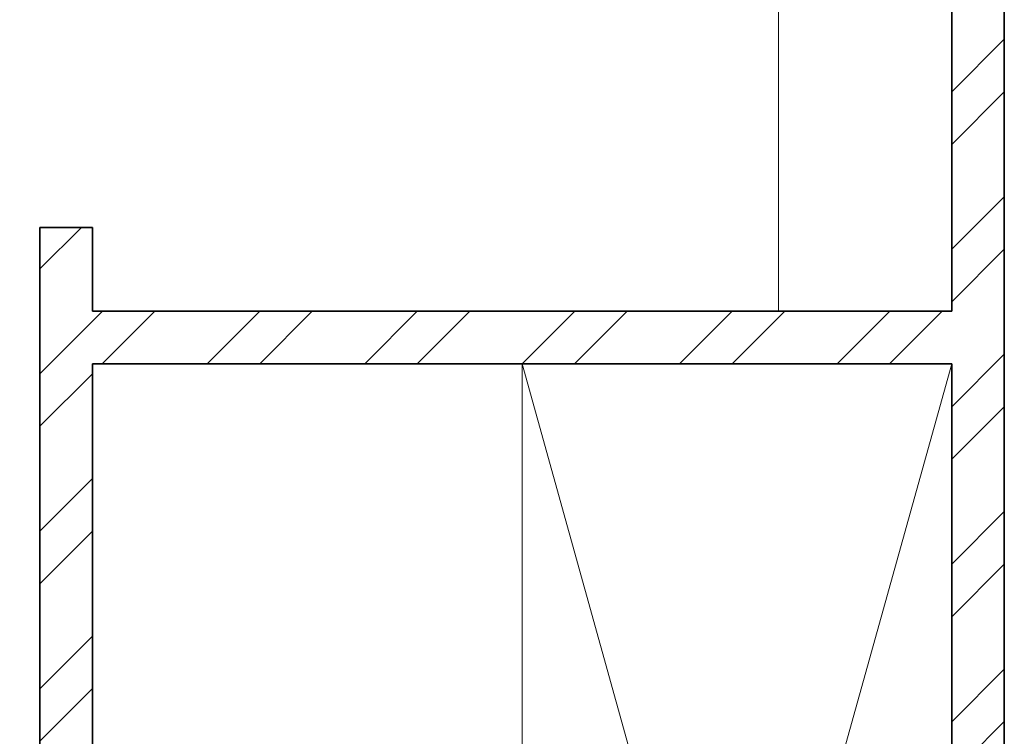
# Model space of a CAD drawing. Units: inches. Extents: x 2168 to 3056, y 1130 to 2629.
# Tile 16 of 42: x 2780 to 2864, y 1956 to 2017. Entities that reach past the tile are written whole.
import ezdxf

# ---------------------------------------------------------------- set-up
doc = ezdxf.new("R2010")
doc.units = ezdxf.units.IN
for name, color, linetype, lineweight in [('A-FLOR-CASE', 71, 'Continuous', 18), ('A-FLOR-OTLN', 7, 'Continuous', 18), ('A-WALL', 7, 'Continuous', 35)]:
    doc.layers.add(name, color=color, linetype=linetype, lineweight=lineweight)
doc.layers.add('A-WALL-PATT', color=143, linetype='Continuous', lineweight=13, true_color=0x7aafdf)

msp = doc.modelspace()

# ---------------------------------------------------------------- hatches: boundary and pattern name
at = {"layer": 'A-WALL-PATT'}
h = msp.add_hatch(dxfattribs=at)
h.set_pattern_fill('ANSI32', color=256)
h.paths.add_polyline_path([(2463.796, 2409.389), (2467.387, 2409.389), (2467.387, 2413.889), (2454.768, 2413.889), (2454.768, 2411.639), (2454.768, 2409.389), (2459.296, 2409.389), (2459.296, 2265.389), (2455.644, 2265.389), (2455.644, 2260.889), (2467.349, 2260.889), (2467.349, 2263.139), (2467.349, 2265.389), (2463.796, 2265.389)])
h.paths.add_polyline_path([(2431.596, 2413.889), (2409.647, 2413.889), (2409.647, 2409.389), (2431.596, 2409.389), (2431.596, 2411.639)])
h.paths.add_polyline_path([(2349.647, 2413.889), (2331.796, 2413.889), (2331.796, 2362.671), (2336.296, 2362.671), (2336.296, 2409.389), (2349.647, 2409.389), (2349.647, 2411.639)])
h.paths.add_polyline_path([(2634.149, 2411.639), (2634.149, 2413.889), (2562.293, 2413.889), (2562.293, 2409.389), (2595.796, 2409.389), (2595.796, 2280.309), (2595.826, 2280.309), (2595.826, 2265.389), (2499.91, 2265.389), (2499.91, 2260.889), (2550.796, 2260.889), (2550.796, 2117.308), (2555.296, 2117.308), (2555.296, 2168.08), (2571.93, 2168.08), (2571.93, 2176.889), (2559.796, 2176.889), (2559.796, 2256.389), (2640.796, 2256.389), (2640.796, 2176.889), (2626.428, 2176.889), (2626.428, 2168.08), (2645.296, 2168.08), (2645.296, 2116.637), (2649.796, 2116.637), (2649.796, 2260.889), (2691.251, 2260.889), (2691.251, 2263.139), (2691.251, 2265.389), (2670.655, 2265.389), (2670.655, 2265.365), (2600.296, 2265.365), (2600.296, 2280.258), (2600.296, 2409.389), (2634.149, 2409.389)])
h.paths.add_polyline_path([(2600.296, 2473.889), (2612.84, 2473.889), (2612.84, 2478.389), (2572.636, 2478.389), (2572.636, 2473.889), (2595.796, 2473.889), (2595.796, 2413.889), (2600.296, 2413.889)])
h.paths.add_polyline_path([(2535.796, 2473.889), (2548.636, 2473.889), (2548.636, 2478.389), (2531.396, 2478.389), (2531.396, 2413.889), (2521.6, 2413.889), (2521.6, 2409.389), (2539.239, 2409.389), (2539.239, 2411.639), (2539.239, 2413.889), (2535.796, 2413.889)])
h.paths.add_polyline_path([(2664.796, 2478.389), (2636.84, 2478.389), (2636.84, 2473.889), (2660.296, 2473.889), (2660.296, 2413.889), (2656.165, 2413.889), (2656.165, 2409.389), (2671.684, 2409.389), (2671.684, 2411.639), (2671.684, 2413.889), (2664.796, 2413.889)])
h.paths.add_polyline_path([(2705.942, 2413.889), (2695.684, 2413.889), (2695.684, 2409.389), (2705.942, 2409.389)])
h.paths.add_polyline_path([(2741.35, 2413.889), (2728.733, 2413.889), (2728.733, 2411.639), (2728.733, 2409.389), (2732.296, 2409.389), (2732.296, 2265.389), (2725.733, 2265.389), (2725.733, 2260.889), (2740.917, 2260.889), (2740.917, 2263.139), (2740.917, 2265.389), (2736.796, 2265.389), (2736.796, 2409.389), (2741.35, 2409.389)])
h.paths.add_polyline_path([(2785.655, 2413.889), (2764.546, 2413.889), (2764.486, 2409.389), (2785.655, 2409.389), (2785.655, 2411.639)])
h.paths.add_polyline_path([(2864.296, 2413.889), (2845.655, 2413.889), (2845.655, 2409.389), (2859.796, 2409.389), (2859.796, 2368.425), (2864.296, 2368.425)])
h.paths.add_polyline_path([(2864.296, 2308.425), (2862.046, 2308.425), (2859.796, 2308.425), (2859.796, 2265.389), (2774.483, 2265.389), (2774.483, 2263.139), (2774.483, 2260.889), (2781.796, 2260.889), (2781.796, 2226.654), (2786.296, 2226.654), (2786.296, 2260.889), (2859.796, 2260.889), (2859.796, 2241.352), (2864.296, 2241.352)])
h.paths.add_polyline_path([(2864.296, 2217.352), (2862.046, 2217.352), (2859.796, 2217.352), (2859.796, 2200.889), (2786.296, 2200.889), (2786.296, 2205.931), (2784.046, 2205.931), (2781.796, 2205.931), (2781.796, 2150.974), (2786.296, 2150.974), (2786.296, 2161.889), (2859.796, 2161.889), (2859.796, 2144.419), (2864.296, 2144.419)])
h.paths.add_polyline_path([(2859.796, 2196.389), (2859.796, 2166.389), (2786.296, 2166.389), (2786.296, 2196.389)], flags=16)
h.paths.add_polyline_path([(2864.296, 2108.419), (2862.046, 2108.419), (2859.796, 2108.419), (2859.796, 2080.889), (2786.296, 2080.889), (2786.296, 2111.993), (2781.796, 2111.993), (2781.796, 2080.889), (2649.796, 2080.889), (2649.796, 2086.036), (2647.546, 2086.036), (2645.296, 2086.036), (2645.296, 2071.739), (2649.796, 2071.739), (2649.796, 2076.389), (2781.796, 2076.389), (2781.796, 2041.792), (2786.296, 2041.792), (2786.296, 2076.389), (2859.796, 2076.389), (2859.796, 2058.577), (2864.296, 2058.577)])
h.paths.add_polyline_path([(2864.296, 2022.577), (2859.796, 2022.577), (2859.796, 1992.389), (2786.296, 1992.389), (2786.296, 1999.573), (2781.796, 1999.573), (2781.796, 1848.085), (2784.046, 1848.085), (2786.296, 1848.085), (2786.296, 1851.389), (2859.796, 1851.389), (2859.796, 1838.258), (2864.296, 1838.258)], flags=17)
h.paths.add_polyline_path([(2859.796, 1987.889), (2859.796, 1855.889), (2786.296, 1855.889), (2786.296, 1987.889)], flags=16)
h.paths.add_polyline_path([(2823.046, 1987.889), (2841.421, 1921.889), (2823.046, 1855.889)], flags=0)
h.paths.add_polyline_path([(2864.296, 1814.258), (2859.796, 1814.258), (2859.796, 1791.389), (2786.296, 1791.389), (2786.296, 1825.658), (2784.046, 1825.658), (2781.796, 1825.658), (2781.796, 1791.389), (2720.155, 1791.389), (2720.155, 1791.265), (2649.796, 1791.265), (2649.796, 1806.159), (2649.796, 2038.983), (2647.546, 2038.983), (2645.296, 2038.983), (2645.296, 1783.925), (2649.796, 1783.925), (2649.796, 1786.889), (2781.796, 1786.889), (2781.796, 1746.789), (2786.296, 1746.789), (2786.296, 1786.889), (2859.796, 1786.889), (2859.796, 1770.083), (2864.296, 1770.083)])
h.paths.add_polyline_path([(2864.296, 1734.083), (2862.046, 1734.083), (2859.796, 1734.083), (2859.796, 1705.889), (2786.296, 1705.889), (2786.296, 1714.166), (2781.796, 1714.166), (2781.796, 1660.527), (2786.296, 1660.527), (2786.296, 1666.889), (2859.796, 1666.889), (2859.796, 1648.342), (2864.296, 1648.342)])
h.paths.add_polyline_path([(2786.296, 1701.389), (2859.796, 1701.389), (2859.796, 1671.389), (2786.296, 1671.389)], flags=16)
h.paths.add_polyline_path([(2649.796, 1756.576), (2647.546, 1756.576), (2645.296, 1756.576), (2645.296, 1606.889), (2555.296, 1606.889), (2555.296, 1749.513), (2553.046, 1749.513), (2550.796, 1749.513), (2550.796, 1606.889), (2503.006, 1606.889), (2503.006, 1604.639), (2503.006, 1602.389), (2595.796, 1602.389), (2595.849, 1602.389), (2595.849, 1587.495), (2595.796, 1458.389), (2561.502, 1458.389), (2561.502, 1456.139), (2561.502, 1453.889), (2595.796, 1453.889), (2595.796, 1381.889), (2573.438, 1381.889), (2573.438, 1377.389), (2613.01, 1377.389), (2613.01, 1379.639), (2613.01, 1381.889), (2600.296, 1381.889), (2600.296, 1453.889), (2634.327, 1453.889), (2634.327, 1458.389), (2600.296, 1458.389), (2600.296, 1602.389), (2670.655, 1602.389), (2694.095, 1602.389), (2694.095, 1606.889), (2649.796, 1606.889)])
h.paths.add_polyline_path([(2736.796, 1602.389), (2741.562, 1602.389), (2741.562, 1606.889), (2726.203, 1606.889), (2726.203, 1604.639), (2726.203, 1602.389), (2732.296, 1602.389), (2732.296, 1458.389), (2727.899, 1458.389), (2727.899, 1453.889), (2740.821, 1453.889), (2740.821, 1456.139), (2740.821, 1458.389), (2736.796, 1458.389)])
h.paths.add_polyline_path([(2859.796, 1606.889), (2786.296, 1606.889), (2786.296, 1637.334), (2784.046, 1637.334), (2781.796, 1637.334), (2781.796, 1606.889), (2775.612, 1606.889), (2775.612, 1602.389), (2859.796, 1602.389)])
h.paths.add_polyline_path([(2864.296, 1624.342), (2862.046, 1624.342), (2859.796, 1624.342), (2859.796, 1570.39), (2864.296, 1570.39)])
h.paths.add_polyline_path([(2864.296, 1510.39), (2862.046, 1510.39), (2859.796, 1510.39), (2859.796, 1458.389), (2846.735, 1458.389), (2846.735, 1456.139), (2846.735, 1453.889), (2864.296, 1453.889)])
h.paths.add_polyline_path([(2786.735, 1458.389), (2765.444, 1458.389), (2765.444, 1453.889), (2786.735, 1453.889)])
h.paths.add_polyline_path([(2706.004, 1458.389), (2695.36, 1458.389), (2695.36, 1453.889), (2706.004, 1453.889), (2706.004, 1456.139)])
h.paths.add_polyline_path([(2671.36, 1456.139), (2671.36, 1458.389), (2655.986, 1458.389), (2655.986, 1456.139), (2655.986, 1453.889), (2660.296, 1453.889), (2660.296, 1381.889), (2637.01, 1381.889), (2637.01, 1377.389), (2664.796, 1377.389), (2664.796, 1453.889), (2671.36, 1453.889)], flags=17)
h.paths.add_polyline_path([(2539.829, 1458.389), (2520.237, 1458.389), (2520.237, 1453.889), (2531.296, 1453.889), (2531.296, 1377.389), (2546.449, 1377.389), (2546.449, 1379.639), (2546.449, 1381.889), (2535.796, 1381.889), (2535.796, 1453.889), (2539.829, 1453.889)], flags=17)
h.paths.add_polyline_path([(2496.237, 1458.389), (2489.13, 1458.389), (2489.13, 1453.889), (2496.237, 1453.889), (2496.237, 1456.139)])
h.paths.add_polyline_path([(2467.433, 1456.139), (2467.433, 1458.389), (2463.796, 1458.389), (2463.796, 1602.389), (2468.242, 1602.389), (2468.242, 1605.7), (2468.242, 1606.889), (2454.602, 1606.889), (2454.602, 1602.389), (2459.296, 1602.389), (2459.296, 1458.389), (2454.24, 1458.389), (2454.24, 1453.889), (2467.433, 1453.889)])
h.paths.add_polyline_path([(2431.601, 1456.139), (2431.601, 1458.389), (2411.386, 1458.389), (2411.386, 1453.889), (2431.601, 1453.889)])
h.paths.add_polyline_path([(2351.386, 1458.389), (2336.296, 1458.389), (2336.296, 1490.693), (2334.046, 1490.693), (2331.796, 1490.693), (2331.796, 1453.889), (2351.386, 1453.889), (2351.386, 1456.139)])
h.paths.add_polyline_path([(2336.296, 1629.705), (2331.796, 1629.705), (2331.796, 1552.317), (2336.296, 1552.317), (2336.296, 1602.389), (2406.655, 1602.389), (2423.472, 1602.389), (2423.472, 1606.889), (2418.796, 1606.889), (2418.796, 1643.678), (2416.546, 1643.678), (2414.296, 1643.678), (2414.296, 1606.889), (2336.296, 1606.889)])
h.paths.add_polyline_path([(2418.796, 1714.384), (2414.296, 1714.384), (2414.296, 1705.889), (2336.296, 1705.889), (2336.296, 1731.324), (2334.046, 1731.324), (2331.796, 1731.324), (2331.796, 1653.705), (2334.046, 1653.705), (2336.296, 1653.705), (2336.296, 1666.889), (2414.296, 1666.889), (2414.296, 1663.589), (2418.796, 1663.589)])
h.paths.add_polyline_path([(2336.296, 1701.389), (2414.296, 1701.389), (2414.296, 1671.389), (2336.296, 1671.389)], flags=16)
h.paths.add_polyline_path([(2555.296, 2040.059), (2550.796, 2040.059), (2550.796, 1791.389), (2550.561, 1791.205), (2480.202, 1791.205), (2418.796, 1791.389), (2418.796, 1825.448), (2416.546, 1825.448), (2414.296, 1825.448), (2414.296, 1791.389), (2336.296, 1791.389), (2336.296, 1806.409), (2331.796, 1806.409), (2331.796, 1767.324), (2336.296, 1767.324), (2336.296, 1786.889), (2414.296, 1786.889), (2414.296, 1745.457), (2418.796, 1745.457), (2418.796, 1786.889), (2550.796, 1786.889), (2550.796, 1783.011), (2555.296, 1783.011)])
h.paths.add_polyline_path([(2418.796, 1923.389), (2423.207, 1923.389), (2423.207, 1925.639), (2423.207, 1927.889), (2418.796, 1927.889), (2418.796, 2000.048), (2414.296, 2000.048), (2414.296, 1992.389), (2336.296, 1992.389), (2336.296, 1987.889), (2414.296, 1987.889), (2414.296, 1855.889), (2336.296, 1855.889), (2336.296, 1851.389), (2414.296, 1851.389), (2414.296, 1846.759), (2418.796, 1846.759)], flags=17)
h.paths.add_polyline_path([(2336.296, 2019.294), (2334.046, 2019.294), (2331.796, 2019.294), (2331.796, 1830.409), (2336.296, 1830.409)], flags=17)
h.paths.add_polyline_path([(2550.796, 1927.889), (2453.541, 1927.889), (2453.541, 1925.639), (2453.541, 1923.389), (2550.796, 1923.389)], flags=17)
h.paths.add_polyline_path([(2744.987, 1927.889), (2649.796, 1927.889), (2649.796, 1923.389), (2744.987, 1923.389), (2744.987, 1925.639)], flags=17)
h.paths.add_polyline_path([(2555.296, 2086.458), (2553.046, 2086.458), (2550.796, 2086.458), (2550.796, 2080.889), (2418.796, 2080.889), (2336.296, 2080.889), (2336.296, 2115.399), (2334.046, 2115.399), (2331.796, 2115.399), (2331.796, 2055.294), (2336.296, 2055.294), (2336.296, 2076.389), (2550.796, 2076.389), (2550.796, 2071.538), (2555.296, 2071.538)])
h.paths.add_polyline_path([(2418.796, 2121.389), (2414.296, 2121.389), (2414.296, 2080.889), (2418.796, 2080.889)])
h.paths.add_polyline_path([(2418.796, 2076.389), (2414.296, 2076.389), (2414.296, 2035.123), (2418.796, 2035.123)])
h.paths.add_polyline_path([(2422.868, 2263.139), (2422.868, 2265.389), (2406.655, 2265.389), (2406.655, 2265.359), (2336.296, 2265.359), (2336.296, 2280.252), (2336.296, 2302.671), (2334.046, 2302.671), (2331.796, 2302.671), (2331.796, 2246.853), (2336.296, 2246.853), (2336.296, 2260.889), (2414.296, 2260.889), (2414.296, 2223.996), (2418.796, 2223.996), (2418.796, 2260.889), (2422.868, 2260.889)])
h.paths.add_polyline_path([(2418.796, 2204.783), (2416.546, 2204.783), (2414.296, 2204.783), (2414.296, 2200.889), (2336.296, 2200.889), (2336.296, 2220.853), (2331.796, 2220.853), (2331.796, 2151.399), (2336.296, 2151.399), (2336.296, 2161.889), (2414.296, 2161.889), (2414.296, 2153.726), (2418.796, 2153.726)])
h.paths.add_polyline_path([(2414.296, 2196.389), (2414.296, 2166.389), (2336.296, 2166.389), (2336.296, 2196.389)], flags=16)
h.paths.add_polyline_path([(2375.296, 2181.389), (2336.296, 2166.389), (2336.296, 2196.389)], flags=0)
h.paths.add_polyline_path([(2809.595, 2172.34), (2838.804, 2172.34), (2838.804, 2190.997), (2809.595, 2190.997)], flags=8)
h.paths.add_polyline_path([(2849.75, 1919.585), (2849.75, 1952.672), (2831.093, 1952.672), (2831.093, 1919.585)], flags=8)
h.paths.add_polyline_path([(2808.875, 1901.967), (2808.875, 1937.85), (2790.149, 1937.85), (2790.149, 1901.967)], flags=8)
h.paths.add_polyline_path([(2806.285, 1671.896), (2835.493, 1671.896), (2835.493, 1690.553), (2806.285, 1690.553)], flags=8)
h.paths.add_polyline_path([(2353.186, 1676.549), (2382.395, 1676.549), (2382.395, 1695.207), (2353.186, 1695.207)], flags=8)
h.paths.add_polyline_path([(2360.083, 1832.308), (2389.241, 1832.308), (2389.241, 1850.966), (2360.083, 1850.966)], flags=25)
h.paths.add_polyline_path([(2354.822, 2167.823), (2384.031, 2167.823), (2384.031, 2186.481), (2354.822, 2186.481)], flags=8)

# ---------------------------------------------------------------- linework, layer by layer
at = {"layer": 'A-FLOR-CASE'}
msp.add_line((2844.993, 2059.09), (2844.993, 1992.389), dxfattribs=at)
at = {"layer": 'A-FLOR-OTLN'}
for p, q in [((2823.046, 1987.889), (2823.046, 1855.889)), ((2823.046, 1855.889), (2859.796, 1987.889)), ((2823.046, 1987.889), (2859.796, 1855.889))]:
    msp.add_line(p, q, dxfattribs=at)
at = {"layer": 'A-WALL'}
for p, q in [((2859.796, 2022.577), (2859.796, 1992.389)), ((2864.296, 2022.577), (2864.296, 1838.258)), ((2781.796, 1999.573), (2786.296, 1999.573)), ((2781.796, 1999.573), (2781.796, 1848.085)), ((2786.296, 1999.573), (2786.296, 1992.389)), ((2786.296, 1992.389), (2859.796, 1992.389)), ((2786.296, 1987.889), (2859.796, 1987.889)), ((2786.296, 1987.889), (2786.296, 1855.889)), ((2859.796, 1987.889), (2859.796, 1855.889))]:
    msp.add_line(p, q, dxfattribs=at)

doc.saveas('drawing.dxf')
